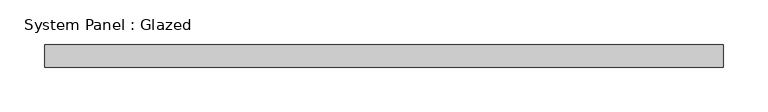
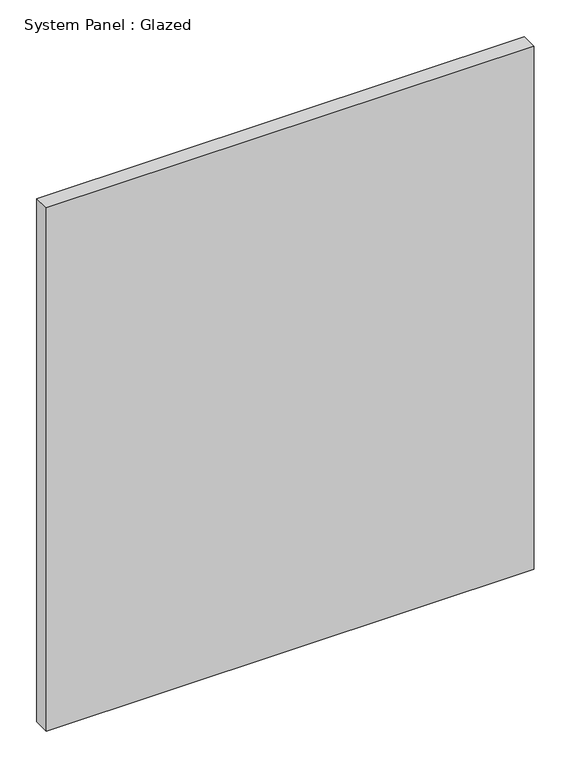
"""IFC4 building model written with IfcOpenShell, lengths in millimetres: plate geometry, System Panel : Glazed."""

from ifc_helpers import new_model, si_unit, origin, origin_with_axes, place, context, project, spatial, polyline, outline, extrude, source, transform, mapped, element, save


def system_panel_glazed_10c9008b(model_context):
    return source(origin(), model_context, "Body", "SweptSolid", [
        extrude(outline(polyline([(381.0, 19.05), (-381.0, 19.05), (-381.0, 44.45), (381.0, 44.45), (381.0, 19.05)])), origin_with_axes(), (0.0, 0.0, 1.0), 863.6),
    ])


if __name__ == "__main__":
    model = new_model("IFC4")
    model_context = context("Model", 3, world=origin())
    ifc_project = project(units=[si_unit("LENGTHUNIT", "METRE", prefix="MILLI")], contexts=[model_context])
    site = spatial("IfcSite", under=ifc_project)
    building = spatial("IfcBuilding", under=site)
    placement = place(None, origin())
    system_panel_glazed_shape = system_panel_glazed_10c9008b(model_context)
    element("IfcPlate", 1, ObjectType="System Panel : Glazed", at=placement, inside=building, context=model_context, shape_type="MappedRepresentation", body=[
        mapped(system_panel_glazed_shape, transform((0.0, 0.0, 0.0), x_axis=(1.0, 0.0, 0.0), y_axis=(0.0, 1.0, 0.0), z_axis=(0.0, 0.0, 1.0))),
    ])
    save(model, "model.ifc")

# Revit data of these elements
# Type "System Panel : Glazed"
#   Construction Type Id = "GSP4R"
#   Analytic Construction = "1/8 in Pilkington single glazing"
#   Visual Light Transmittance = 0.9
#   Solar Heat Gain Coefficient = 0.86
#   Heat Transfer Coefficient (U) = 1.18115 BTU/(h·ft²·°F)
# Element 1 (IfcPlate, "System Panel : Glazed")
#   Materials on its faces: "Glass"
# Materials
#   "Glass": class "Glass", colour RGB 0 128 192, transparency 0.75, Description = "Soda Lime Glass", Cost = 0
